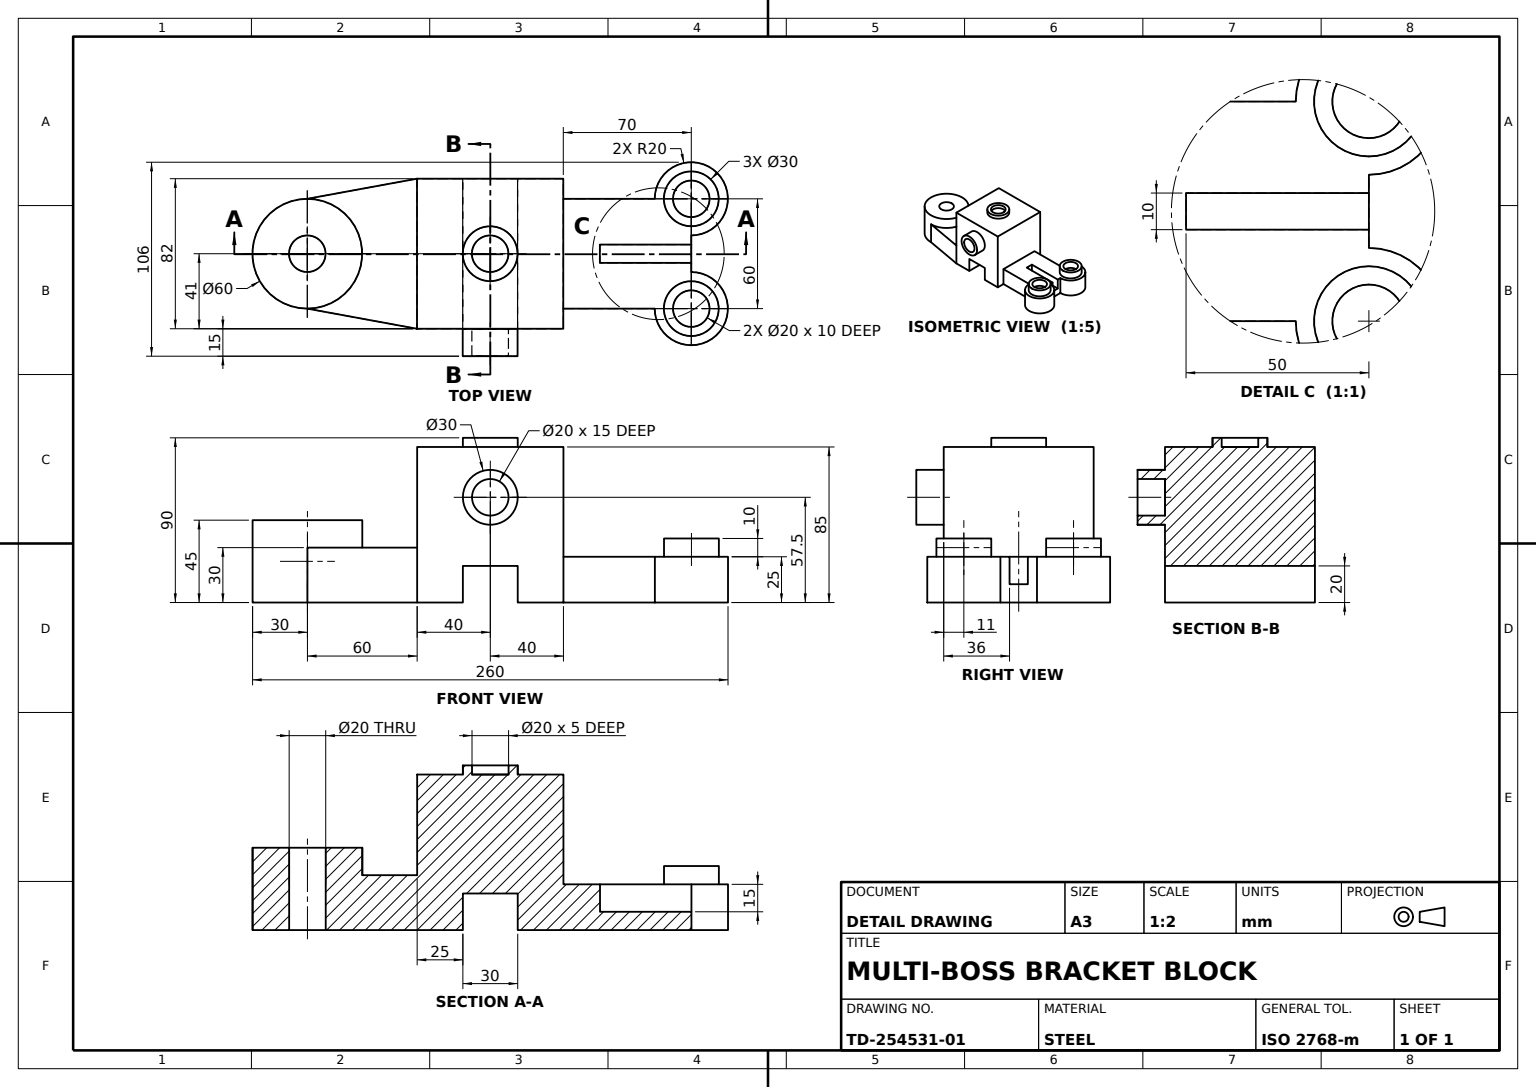
from build123d import *

# Parameters (mm, degrees)
MAIN_BLOCK_DEPTH          = 82
SIDE_LUG_PROFILE_R        = 30
SIDE_LUG_PROFILE_R_2      = 10
SIDE_LUG_BOSS_DEPTH       = 45
GUSSET_BOSS_DEPTH         = 30
MOUNTING_TAB_PROFILE_W    = 70
MOUNTING_TAB_PROFILE_H    = 60
MOUNTING_TAB_DEPTH        = 25
TAB_EYE_PROFILE_R         = 20
TAB_EYE_BOSS_DEPTH        = 25
TAB_RING_PROFILES_R       = 15
TAB_RING_PROFILES_R_2     = 10
TAB_BOSS_RINGS_DEPTH      = 10
SIDE_HUB_RING_PROFILE_R   = 15
SIDE_HUB_RING_PROFILE_R_2 = 10
SIDE_HUB_RING_DEPTH       = 5
TOP_HUB_RING_PROFILE_R    = 15
TOP_HUB_RING_PROFILE_R_2  = 10
TOP_HUB_RING_DEPTH        = 15
TAB_SLOT_CUT_DEPTH        = 15


with BuildPart() as part:
    # Main Block Profile → Main Block (new body)
    with BuildSketch(Plane.XY):
        Polygon((0, 0), (25, 0), (25, 20), (55, 20), (55, 0), (80, 0), (80, 85), (0, 85), align=None)
    extrude(amount=MAIN_BLOCK_DEPTH)



with BuildPart() as body_2:
    # Side Lug Profile → Side Lug Boss (new body)
    with BuildSketch(Plane(origin=(0, 0, 0), x_dir=(1, 0, 0), z_dir=(0, 1, 0))):
        with Locations(Location((-60, -41, 0), (0, 0, 90))):
            Circle(SIDE_LUG_PROFILE_R)
        with Locations(Location((-60, -41, 0), (0, 0, 90))):
            Circle(SIDE_LUG_PROFILE_R_2, mode=Mode.SUBTRACT)
    extrude(amount=SIDE_LUG_BOSS_DEPTH)


with BuildPart() as part_1:
    add(part.part)

    add(body_2.part)  # Gusset Boss merges body 2
    # Gusset Profile → Gusset Boss (add)
    with BuildSketch(Plane(origin=(0, 0, 0), x_dir=(1, 0, 0), z_dir=(0, 1, 0))):
        with BuildLine():
            Line((0, 0), (-60, -11))
            ThreePointArc((-60, -11), (-30, -41), (-60, -71))
            Line((-60, -71), (0, -82))
            Line((0, -82), (0, 0))
        make_face()
    extrude(amount=GUSSET_BOSS_DEPTH)

    # Mounting Tab Profile → Mounting Tab (add)
    with BuildSketch(Plane(origin=(0, 0, 0), x_dir=(1, 0, 0), z_dir=(0, 1, 0))):
        with Locations((115, -41)):
            Rectangle(MOUNTING_TAB_PROFILE_W, MOUNTING_TAB_PROFILE_H)
    extrude(amount=MOUNTING_TAB_DEPTH)

    # Tab Eye Profile → Tab Eye Boss (add)
    with BuildSketch(Plane(origin=(0, 25, 0), x_dir=(1, 0, 0), z_dir=(0, 1, 0))):
        with Locations((150, -11)):
            Circle(TAB_EYE_PROFILE_R)
        with Locations((150, -71)):
            Circle(TAB_EYE_PROFILE_R)
    extrude(amount=-TAB_EYE_BOSS_DEPTH)

    # Tab Ring Profiles → Tab Boss Rings (add)
    # profile 1 of 2: a face of its own
    with BuildSketch(Plane(origin=(0, 25, 0), x_dir=(1, 0, 0), z_dir=(0, 1, 0))):
        with Locations(Location((150, -11, 0), (0, 0, 90))):
            Circle(TAB_RING_PROFILES_R)
        with Locations(Location((150, -11, 0), (0, 0, 270))):
            Circle(TAB_RING_PROFILES_R_2, mode=Mode.SUBTRACT)
    # profile 2 of 2: a face of its own
    with BuildSketch(Plane(origin=(0, 25, 0), x_dir=(1, 0, 0), z_dir=(0, 1, 0))):
        with Locations(Location((150, -71, 0), (0, 0, 90))):
            Circle(TAB_RING_PROFILES_R)
        with Locations(Location((150, -71, 0), (0, 0, 270))):
            Circle(TAB_RING_PROFILES_R_2, mode=Mode.SUBTRACT)
    extrude(amount=TAB_BOSS_RINGS_DEPTH)

    # Side Hub Ring Profile → Side Hub Ring (add)
    with BuildSketch(Plane(origin=(0, 85, 0), x_dir=(1, 0, 0), z_dir=(0, 1, 0))):
        with Locations((40, -41)):
            Circle(SIDE_HUB_RING_PROFILE_R)
        with Locations(Location((40, -41, 0), (0, 0, 180))):
            Circle(SIDE_HUB_RING_PROFILE_R_2, mode=Mode.SUBTRACT)
    extrude(amount=SIDE_HUB_RING_DEPTH)

    # Top Hub Ring Profile → Top Hub Ring (add)
    with BuildSketch(Plane.XY.offset(82)):
        with Locations((40, 57.5)):
            Circle(TOP_HUB_RING_PROFILE_R)
        with Locations((40, 57.5)):
            Circle(TOP_HUB_RING_PROFILE_R_2, mode=Mode.SUBTRACT)
    extrude(amount=TOP_HUB_RING_DEPTH)

    # Tab Slot Profile → Tab Slot Cut (cut)
    with BuildSketch(Plane(origin=(0, 25, 0), x_dir=(1, 0, 0), z_dir=(0, 1, 0))):
        Polygon((150, -41), (150, -36), (100, -36), (100, -46), (150, -46), align=None)
    extrude(amount=-TAB_SLOT_CUT_DEPTH, mode=Mode.SUBTRACT)


solid = part_1.part
